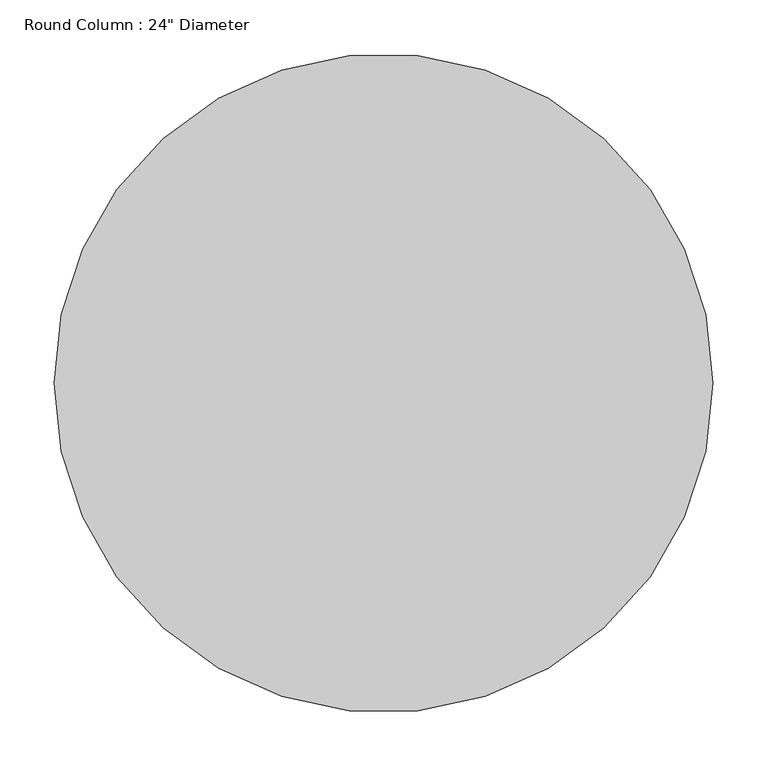
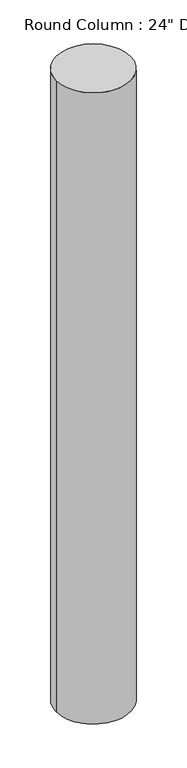
"""IFC4 building model written with IfcOpenShell, lengths in millimetres: column geometry."""

from ifc_helpers import new_model, si_unit, point, frame, frame_2d, origin, place, context, project, spatial, circle_curve, trimmed, segment, composite_curve, outline, extrude, source, transform, mapped, element, save


def column_dfe452ed(model_context):
    return source(origin(), model_context, "Body", "SweptSolid", [
        extrude(outline(composite_curve([segment(trimmed(circle_curve(frame_2d((3142.4703248, 4403.9959709)), 304.8), [point((2837.6703248, 4403.9959709))], [point((3447.2703248, 4403.9959709))], False, "CARTESIAN"), True, "CONTINUOUS"), segment(trimmed(circle_curve(frame_2d((3142.4703248, 4403.9959709)), 304.8), [point((3447.2703248, 4403.9959709))], [point((2837.6703248, 4403.9959709))], False, "CARTESIAN"), True, "CONTINUOUS")], self_intersect=False)), frame((0.0, 0.0, 21031.2), z_axis=(0.0, 0.0, 1.0), x_axis=(1.0, 0.0, 0.0)), (0.0, 0.0, 1.0), 5486.4),
    ])


if __name__ == "__main__":
    model = new_model("IFC4")
    model_context = context("Model", 3, world=origin())
    ifc_project = project(units=[si_unit("LENGTHUNIT", "METRE", prefix="MILLI")], contexts=[model_context])
    site = spatial("IfcSite", under=ifc_project)
    building = spatial("IfcBuilding", under=site)
    placement = place(None, origin())
    column_shape = column_dfe452ed(model_context)
    element("IfcColumn", 1, ObjectType="Round Column : 24\" Diameter", at=placement, inside=building, context=model_context, shape_type="MappedRepresentation", body=[
        mapped(column_shape, transform((0.0, 0.0, 0.0), x_axis=(1.0, 0.0, 0.0), y_axis=(0.0, 1.0, 0.0), z_axis=(0.0, 0.0, 1.0))),
    ])
    save(model, "model.ifc")

# Revit data of these elements
# Type "Round Column : 24\" Diameter"
#   Assembly Code = "B1010200"
#   Diameter = 2' - 0"
#   Offset Base = 0' - 0"
#   Offset Top = 0' - 0"
#   Material = none
